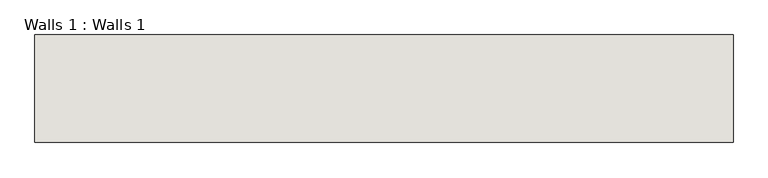
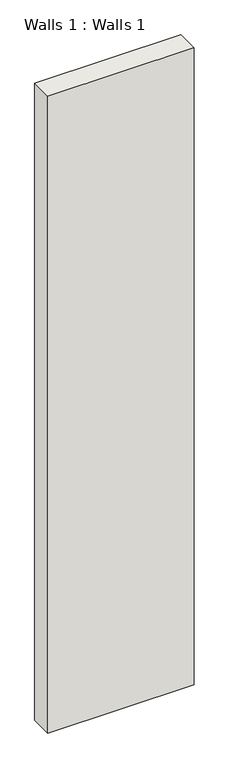
"""IFC4 building model written with IfcOpenShell, lengths in millimetres: wall geometry, Walls 1 : Walls 1."""

from ifc_helpers import new_model, si_unit, origin, origin_with_axes, place, context, project, spatial, polyline, outline, extrude, source, transform, mapped, element, save


def walls_1_walls_1_5577fd9e(model_context):
    return source(origin(), model_context, "Body", "SweptSolid", [
        extrude(outline(polyline([(-4193.9407032, 3556.1956099), (-6175.1407032, 3556.1956099), (-6175.1407032, 3860.9956099), (-4193.9407032, 3860.9956099), (-4193.9407032, 3556.1956099)])), origin_with_axes(), (0.0, 0.0, 1.0), 9118.6695108),
    ])


if __name__ == "__main__":
    model = new_model("IFC4")
    model_context = context("Model", 3, world=origin())
    ifc_project = project(units=[si_unit("LENGTHUNIT", "METRE", prefix="MILLI")], contexts=[model_context])
    site = spatial("IfcSite", under=ifc_project)
    building = spatial("IfcBuilding", under=site)
    placement = place(None, origin())
    walls_1_walls_1_shape = walls_1_walls_1_5577fd9e(model_context)
    element("IfcWall", 1, ObjectType="Walls 1 : Walls 1", at=placement, inside=building, context=model_context, shape_type="MappedRepresentation", body=[
        mapped(walls_1_walls_1_shape, transform((0.0, 0.0, 0.0), x_axis=(1.0, 0.0, 0.0), y_axis=(0.0, 1.0, 0.0), z_axis=(0.0, 0.0, 1.0))),
    ])
    save(model, "model.ifc")

# Revit data of these elements
# Element 1 (IfcWall, "Walls 1 : Walls 1")
#   Materials on its faces: "Default Wall"
# Materials
#   "Default Wall": colour RGB 80 80 80, transparency 0
